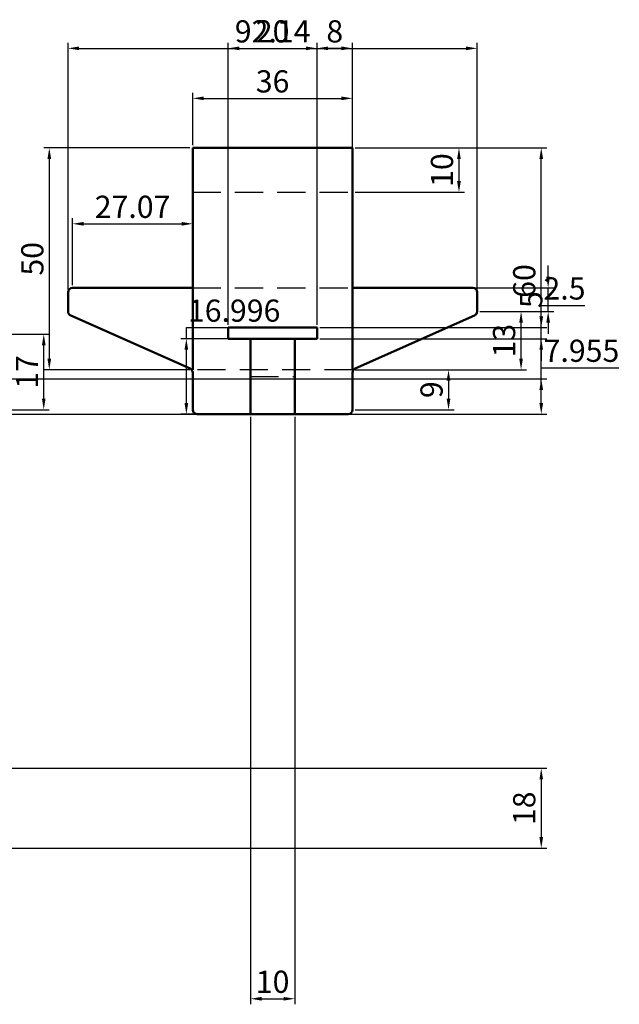
# Model space of a CAD drawing. Units: millimetres. Extents: x 2010 to 2347, y 1200 to 1429.
# Tile 3 of 3: x 2212 to 2347, y 1200 to 1422. Entities that reach past the tile are written whole.
import ezdxf

# ---------------------------------------------------------------- set-up
doc = ezdxf.new("R2010")
doc.units = ezdxf.units.MM
doc.linetypes.add('HIDDEN', pattern=[9.525, 6.35, -3.175])
for name, color, linetype, lineweight in [('M-DIMS', 2, 'Continuous', 25), ('M-HIDN', 3, 'HIDDEN', 25), ('M-OUTL', 7, 'Continuous', 50)]:
    doc.layers.add(name, color=color, linetype=linetype, lineweight=lineweight)
doc.styles.get("Standard").update_dxf_attribs({"font": 'arial.ttf'})
doc.dimstyles.new('ISO-25', dxfattribs={"dimtxt": 5, "dimasz": 2.5, "dimexe": 1.25, "dimexo": 0.625, "dimtad": 1, "dimtoh": 1, "dimdec": 0, "dimtxsty": 'Standard', "dimcen": 2.5, "dimadec": 0, "dimazin": 0, "dimtfac": 1, "dimtdec": 0, "dimtmove": 0, "dimatfit": 3, "dimfxl": 1, "dimarcsym": 0})

# ---------------------------------------------------------------- blocks, each defined once
blk = doc.blocks.new('*D2')
at = {"layer": 'Defpoints', "color": 0, "transparency": 16777216}
for p in [(2196.57, 1351.05), (2217.71, 1351.05), (2197.57, 1334.05)]:
    blk.add_point(p, dxfattribs=at)
at = {"layer": 'M-DIMS', "color": 0, "lineweight": -2, "transparency": 16777216}
for p, q in [((2197.19, 1351.05), (2218.96, 1351.05)), ((2217.71, 1336.55), (2217.71, 1348.55)), ((2198.19, 1334.05), (2218.96, 1334.05))]:
    blk.add_line(p, q, dxfattribs=at)
at = {"layer": 'M-DIMS', "color": 0, "transparency": 16777216}
for points in [[(2217.3, 1348.55), (2218.13, 1348.55), (2217.71, 1351.05)], [(2217.3, 1336.55), (2218.13, 1336.55), (2217.71, 1334.05)]]:
    blk.add_solid(points, dxfattribs=at)
at = {"layer": 'M-DIMS', "color": 0, "transparency": 16777216, "insert": (2214.58, 1342.55), "char_height": 5, "attachment_point": 5, "rotation": 90}
blk.add_mtext('17', dxfattribs=at)
blk = doc.blocks.new('*D17')
at = {"layer": 'Defpoints', "color": 0, "transparency": 16777216}
for p in [(2287.26, 1343.05), (2287.26, 1334.05), (2308.88, 1334.05)]:
    blk.add_point(p, dxfattribs=at)
at = {"layer": 'M-DIMS', "color": 0, "lineweight": -2, "transparency": 16777216}
for p, q in [((2287.89, 1343.05), (2310.13, 1343.05)), ((2308.88, 1340.55), (2308.88, 1336.55)), ((2287.89, 1334.05), (2310.13, 1334.05))]:
    blk.add_line(p, q, dxfattribs=at)
at = {"layer": 'M-DIMS', "color": 0, "transparency": 16777216}
for points in [[(2308.46, 1340.55), (2309.3, 1340.55), (2308.88, 1343.05)], [(2308.46, 1336.55), (2309.3, 1336.55), (2308.88, 1334.05)]]:
    blk.add_solid(points, dxfattribs=at)
at = {"layer": 'M-DIMS', "color": 0, "transparency": 16777216, "insert": (2305.7, 1338.55), "char_height": 5, "attachment_point": 5, "rotation": 90}
blk.add_mtext('9', dxfattribs=at)
blk = doc.blocks.new('*D18')
at = {"layer": 'Defpoints', "color": 0, "transparency": 16777216}
for p in [(2315.33, 1356.16), (2325.22, 1356.16), (2287.26, 1343.05)]:
    blk.add_point(p, dxfattribs=at)
at = {"layer": 'M-DIMS', "color": 0, "lineweight": -2, "transparency": 16777216}
for p, q in [((2315.96, 1356.16), (2326.47, 1356.16)), ((2325.22, 1345.55), (2325.22, 1353.66)), ((2287.89, 1343.05), (2326.47, 1343.05))]:
    blk.add_line(p, q, dxfattribs=at)
at = {"layer": 'M-DIMS', "color": 0, "transparency": 16777216}
for points in [[(2324.8, 1353.66), (2325.63, 1353.66), (2325.22, 1356.16)], [(2324.8, 1345.55), (2325.63, 1345.55), (2325.22, 1343.05)]]:
    blk.add_solid(points, dxfattribs=at)
at = {"layer": 'M-DIMS', "color": 0, "transparency": 16777216, "insert": (2322.04, 1349.6), "char_height": 5, "attachment_point": 5, "rotation": 90}
blk.add_mtext('13', dxfattribs=at)
blk = doc.blocks.new('*D19')
at = {"layer": 'Defpoints', "color": 0, "transparency": 16777216}
for p in [(2314.33, 1361.51), (2331.32, 1361.51), (2315.33, 1356.16)]:
    blk.add_point(p, dxfattribs=at)
at = {"layer": 'M-DIMS', "color": 0, "lineweight": -2, "transparency": 16777216}
for p, q in [((2331.32, 1364.01), (2331.32, 1366.51)), ((2314.96, 1361.51), (2332.57, 1361.51)), ((2331.32, 1356.16), (2331.32, 1361.51)), ((2315.96, 1356.16), (2332.57, 1356.16)), ((2331.32, 1353.66), (2331.32, 1351.16))]:
    blk.add_line(p, q, dxfattribs=at)
at = {"layer": 'M-DIMS', "color": 0, "transparency": 16777216}
for points in [[(2330.9, 1364.01), (2331.73, 1364.01), (2331.32, 1361.51)], [(2330.9, 1353.66), (2331.73, 1353.66), (2331.32, 1356.16)]]:
    blk.add_solid(points, dxfattribs=at)
at = {"layer": 'M-DIMS', "color": 0, "transparency": 16777216, "insert": (2328.15, 1358.84), "char_height": 5, "attachment_point": 5, "rotation": 90}
blk.add_mtext('5', dxfattribs=at)
blk = doc.blocks.new('*D20')
at = {"layer": 'Defpoints', "color": 0, "transparency": 16777216}
for p in [(2287.26, 1393.05), (2287.26, 1383.05), (2311.23, 1383.05)]:
    blk.add_point(p, dxfattribs=at)
at = {"layer": 'M-DIMS', "color": 0, "lineweight": -2, "transparency": 16777216}
for p, q in [((2287.89, 1393.05), (2312.48, 1393.05)), ((2311.23, 1390.55), (2311.23, 1385.55)), ((2287.89, 1383.05), (2312.48, 1383.05))]:
    blk.add_line(p, q, dxfattribs=at)
at = {"layer": 'M-DIMS', "color": 0, "transparency": 16777216}
for points in [[(2310.81, 1390.55), (2311.64, 1390.55), (2311.23, 1393.05)], [(2310.81, 1385.55), (2311.64, 1385.55), (2311.23, 1383.05)]]:
    blk.add_solid(points, dxfattribs=at)
at = {"layer": 'M-DIMS', "color": 0, "transparency": 16777216, "insert": (2308.05, 1388.05), "char_height": 5, "attachment_point": 5, "rotation": 90}
blk.add_mtext('10', dxfattribs=at)
blk = doc.blocks.new('*D21')
at = {"layer": 'Defpoints', "color": 0, "transparency": 16777216}
for p in [(2287.26, 1404.21), (2251.26, 1393.05), (2287.26, 1393.05)]:
    blk.add_point(p, dxfattribs=at)
at = {"layer": 'M-DIMS', "color": 0, "lineweight": -2, "transparency": 16777216}
for p, q in [((2251.26, 1393.67), (2251.26, 1405.46)), ((2287.26, 1393.67), (2287.26, 1405.46)), ((2253.76, 1404.21), (2284.76, 1404.21))]:
    blk.add_line(p, q, dxfattribs=at)
at = {"layer": 'M-DIMS', "color": 0, "transparency": 16777216}
for points in [[(2253.76, 1404.63), (2253.76, 1403.8), (2251.26, 1404.21)], [(2284.76, 1404.63), (2284.76, 1403.8), (2287.26, 1404.21)]]:
    blk.add_solid(points, dxfattribs=at)
at = {"layer": 'M-DIMS', "color": 0, "transparency": 16777216, "insert": (2269.26, 1407.39), "char_height": 5, "attachment_point": 5}
blk.add_mtext('36', dxfattribs=at)
blk = doc.blocks.new('*D22')
at = {"layer": 'Defpoints', "color": 0, "transparency": 16777216}
for p in [(2251.26, 1393.05), (2218.96, 1343.05), (2251.26, 1343.05)]:
    blk.add_point(p, dxfattribs=at)
at = {"layer": 'M-DIMS', "color": 0, "lineweight": -2, "transparency": 16777216}
for p, q in [((2250.64, 1393.05), (2217.71, 1393.05)), ((2218.96, 1390.55), (2218.96, 1345.55)), ((2250.64, 1343.05), (2217.71, 1343.05))]:
    blk.add_line(p, q, dxfattribs=at)
at = {"layer": 'M-DIMS', "color": 0, "transparency": 16777216}
for points in [[(2218.55, 1390.55), (2219.38, 1390.55), (2218.96, 1393.05)], [(2218.55, 1345.55), (2219.38, 1345.55), (2218.96, 1343.05)]]:
    blk.add_solid(points, dxfattribs=at)
at = {"layer": 'M-DIMS', "color": 0, "transparency": 16777216, "insert": (2215.79, 1368.05), "char_height": 5, "attachment_point": 5, "rotation": 90}
blk.add_mtext('50', dxfattribs=at)
blk = doc.blocks.new('*D26')
at = {"layer": 'Defpoints', "color": 0, "transparency": 16777216}
for p in [(2315.33, 1415.48), (2223.19, 1360.51), (2315.33, 1360.51)]:
    blk.add_point(p, dxfattribs=at)
at = {"layer": 'M-DIMS', "color": 0, "lineweight": -2, "transparency": 16777216}
for p, q in [((2223.19, 1361.14), (2223.19, 1416.73)), ((2315.33, 1361.14), (2315.33, 1416.73)), ((2225.69, 1415.48), (2312.83, 1415.48))]:
    blk.add_line(p, q, dxfattribs=at)
at = {"layer": 'M-DIMS', "color": 0, "transparency": 16777216}
for points in [[(2225.69, 1415.9), (2225.69, 1415.06), (2223.19, 1415.48)], [(2312.83, 1415.9), (2312.83, 1415.06), (2315.33, 1415.48)]]:
    blk.add_solid(points, dxfattribs=at)
at = {"layer": 'M-DIMS', "color": 0, "transparency": 16777216, "insert": (2269.26, 1418.66), "char_height": 5, "attachment_point": 5}
blk.add_mtext('92.14', dxfattribs=at)
blk = doc.blocks.new('*D28')
at = {"layer": 'Defpoints', "color": 0, "transparency": 16777216}
for p in [(2279.26, 1415.48), (2259.26, 1352.55), (2279.26, 1352.55)]:
    blk.add_point(p, dxfattribs=at)
at = {"layer": 'M-DIMS', "color": 0, "lineweight": -2, "transparency": 16777216}
for p, q in [((2259.26, 1353.17), (2259.26, 1416.73)), ((2279.26, 1353.17), (2279.26, 1416.73)), ((2261.76, 1415.48), (2276.76, 1415.48))]:
    blk.add_line(p, q, dxfattribs=at)
at = {"layer": 'M-DIMS', "color": 0, "transparency": 16777216}
for points in [[(2261.76, 1415.9), (2261.76, 1415.06), (2259.26, 1415.48)], [(2276.76, 1415.9), (2276.76, 1415.06), (2279.26, 1415.48)]]:
    blk.add_solid(points, dxfattribs=at)
at = {"layer": 'M-DIMS', "color": 0, "transparency": 16777216, "insert": (2269.26, 1418.66), "char_height": 5, "attachment_point": 5}
blk.add_mtext('20', dxfattribs=at)
blk = doc.blocks.new('*D29')
at = {"layer": 'Defpoints', "color": 0, "transparency": 16777216}
for p in [(2264.26, 1333.05), (2274.26, 1333.05), (2274.26, 1201.29)]:
    blk.add_point(p, dxfattribs=at)
at = {"layer": 'M-DIMS', "color": 0, "lineweight": -2, "transparency": 16777216}
for p, q in [((2264.26, 1332.42), (2264.26, 1200.04)), ((2274.26, 1332.42), (2274.26, 1200.04)), ((2266.76, 1201.29), (2271.76, 1201.29))]:
    blk.add_line(p, q, dxfattribs=at)
at = {"layer": 'M-DIMS', "color": 0, "transparency": 16777216}
for points in [[(2266.76, 1201.7), (2266.76, 1200.87), (2264.26, 1201.29)], [(2271.76, 1201.7), (2271.76, 1200.87), (2274.26, 1201.29)]]:
    blk.add_solid(points, dxfattribs=at)
at = {"layer": 'M-DIMS', "color": 0, "transparency": 16777216, "insert": (2269.26, 1204.47), "char_height": 5, "attachment_point": 5}
blk.add_mtext('10', dxfattribs=at)
blk = doc.blocks.new('*D30')
at = {"layer": 'Defpoints', "color": 0, "transparency": 16777216}
for p in [(2279.26, 1352.55), (2329.76, 1352.55), (2279.26, 1350.05)]:
    blk.add_point(p, dxfattribs=at)
at = {"layer": 'M-DIMS', "color": 0, "lineweight": -2, "transparency": 16777216}
for p, q in [((2329.76, 1355.05), (2329.76, 1357.55)), ((2329.76, 1357.55), (2339.61, 1357.55)), ((2279.89, 1352.55), (2331.01, 1352.55)), ((2329.76, 1350.05), (2329.76, 1352.55)), ((2279.89, 1350.05), (2331.01, 1350.05)), ((2329.76, 1347.55), (2329.76, 1345.05))]:
    blk.add_line(p, q, dxfattribs=at)
at = {"layer": 'M-DIMS', "color": 0, "transparency": 16777216}
for points in [[(2329.35, 1355.05), (2330.18, 1355.05), (2329.76, 1352.55)], [(2329.35, 1347.55), (2330.18, 1347.55), (2329.76, 1350.05)]]:
    blk.add_solid(points, dxfattribs=at)
at = {"layer": 'M-DIMS', "color": 0, "transparency": 16777216, "insert": (2335, 1360.72), "char_height": 5, "attachment_point": 5}
blk.add_mtext('2.5', dxfattribs=at)
blk = doc.blocks.new('*D31')
at = {"layer": 'Defpoints', "color": 0, "transparency": 16777216}
for p in [(2249.83, 1350.05), (2264.26, 1350.05), (2264.26, 1333.05)]:
    blk.add_point(p, dxfattribs=at)
at = {"layer": 'M-DIMS', "color": 0, "lineweight": -2, "transparency": 16777216}
for p, q in [((2249.83, 1350.05), (2249.83, 1352.55)), ((2249.83, 1352.55), (2270.74, 1352.55)), ((2263.64, 1350.05), (2248.58, 1350.05)), ((2249.83, 1335.55), (2249.83, 1347.55)), ((2263.64, 1333.05), (2248.58, 1333.05))]:
    blk.add_line(p, q, dxfattribs=at)
at = {"layer": 'M-DIMS', "color": 0, "transparency": 16777216}
for points in [[(2249.41, 1347.55), (2250.25, 1347.55), (2249.83, 1350.05)], [(2249.41, 1335.55), (2250.25, 1335.55), (2249.83, 1333.05)]]:
    blk.add_solid(points, dxfattribs=at)
at = {"layer": 'M-DIMS', "color": 0, "transparency": 16777216, "insert": (2260.6, 1355.72), "char_height": 5, "attachment_point": 5}
blk.add_mtext('16.996', dxfattribs=at)
blk = doc.blocks.new('*D36')
at = {"layer": 'Defpoints', "color": 0, "transparency": 16777216}
for p in [(2106.57, 1341), (2329.76, 1341), (2196.57, 1333.05)]:
    blk.add_point(p, dxfattribs=at)
at = {"layer": 'M-DIMS', "color": 0, "lineweight": -2, "transparency": 16777216}
for p, q in [((2329.76, 1341), (2329.76, 1343.5)), ((2329.76, 1343.5), (2347.26, 1343.5)), ((2107.19, 1341), (2331.01, 1341)), ((2329.76, 1335.55), (2329.76, 1338.5)), ((2197.19, 1333.05), (2331.01, 1333.05))]:
    blk.add_line(p, q, dxfattribs=at)
at = {"layer": 'M-DIMS', "color": 0, "transparency": 16777216}
for points in [[(2329.35, 1338.5), (2330.18, 1338.5), (2329.76, 1341)], [(2329.35, 1335.55), (2330.18, 1335.55), (2329.76, 1333.05)]]:
    blk.add_solid(points, dxfattribs=at)
at = {"layer": 'M-DIMS', "color": 0, "transparency": 16777216, "insert": (2338.82, 1346.68), "char_height": 5, "attachment_point": 5}
blk.add_mtext('7.955', dxfattribs=at)
blk = doc.blocks.new('*D42')
at = {"layer": 'Defpoints', "color": 0, "transparency": 16777216}
for p in [(2287.26, 1393.05), (2329.76, 1393.05), (2286.26, 1333.05)]:
    blk.add_point(p, dxfattribs=at)
at = {"layer": 'M-DIMS', "color": 0, "lineweight": -2, "transparency": 16777216}
for p, q in [((2287.89, 1393.05), (2331.01, 1393.05)), ((2329.76, 1335.55), (2329.76, 1390.55)), ((2286.89, 1333.05), (2331.01, 1333.05))]:
    blk.add_line(p, q, dxfattribs=at)
at = {"layer": 'M-DIMS', "color": 0, "transparency": 16777216}
for points in [[(2329.35, 1390.55), (2330.18, 1390.55), (2329.76, 1393.05)], [(2329.35, 1335.55), (2330.18, 1335.55), (2329.76, 1333.05)]]:
    blk.add_solid(points, dxfattribs=at)
at = {"layer": 'M-DIMS', "color": 0, "transparency": 16777216, "insert": (2326.58, 1363.05), "char_height": 5, "attachment_point": 5, "rotation": 90}
blk.add_mtext('60', dxfattribs=at)
blk = doc.blocks.new('*D43')
at = {"layer": 'Defpoints', "color": 0, "transparency": 16777216}
for p in [(2169.36, 1253.22), (2188.36, 1235.22), (2329.76, 1235.22)]:
    blk.add_point(p, dxfattribs=at)
at = {"layer": 'M-DIMS', "color": 0, "lineweight": -2, "transparency": 16777216}
for p, q in [((2169.98, 1253.22), (2331.01, 1253.22)), ((2329.76, 1250.72), (2329.76, 1237.72)), ((2188.98, 1235.22), (2331.01, 1235.22))]:
    blk.add_line(p, q, dxfattribs=at)
at = {"layer": 'M-DIMS', "color": 0, "transparency": 16777216}
for points in [[(2329.35, 1250.72), (2330.18, 1250.72), (2329.76, 1253.22)], [(2329.35, 1237.72), (2330.18, 1237.72), (2329.76, 1235.22)]]:
    blk.add_solid(points, dxfattribs=at)
at = {"layer": 'M-DIMS', "color": 0, "transparency": 16777216, "insert": (2326.58, 1244.22), "char_height": 5, "attachment_point": 5, "rotation": 90}
blk.add_mtext('18', dxfattribs=at)
blk = doc.blocks.new('*D45')
at = {"layer": 'Defpoints', "color": 0, "transparency": 16777216}
for p in [(2279.26, 1415.48), (2279.26, 1352.55), (2287.26, 1334.05)]:
    blk.add_point(p, dxfattribs=at)
at = {"layer": 'M-DIMS', "color": 0, "lineweight": -2, "transparency": 16777216}
for p, q in [((2279.26, 1353.17), (2279.26, 1416.73)), ((2287.26, 1334.67), (2287.26, 1416.73)), ((2284.76, 1415.48), (2281.76, 1415.48))]:
    blk.add_line(p, q, dxfattribs=at)
at = {"layer": 'M-DIMS', "color": 0, "transparency": 16777216}
for points in [[(2281.76, 1415.9), (2281.76, 1415.06), (2279.26, 1415.48)], [(2284.76, 1415.9), (2284.76, 1415.06), (2287.26, 1415.48)]]:
    blk.add_solid(points, dxfattribs=at)
at = {"layer": 'M-DIMS', "color": 0, "transparency": 16777216, "insert": (2283.26, 1418.66), "char_height": 5, "attachment_point": 5}
blk.add_mtext('8', dxfattribs=at)
blk = doc.blocks.new('*D48')
at = {"layer": 'Defpoints', "color": 0, "transparency": 16777216}
for p in [(2251.26, 1375.94), (2224.19, 1361.51), (2251.26, 1361.51)]:
    blk.add_point(p, dxfattribs=at)
at = {"layer": 'M-DIMS', "color": 0, "lineweight": -2, "transparency": 16777216}
for p, q in [((2224.19, 1362.14), (2224.19, 1377.19)), ((2226.69, 1375.94), (2248.76, 1375.94)), ((2251.26, 1362.14), (2251.26, 1377.19))]:
    blk.add_line(p, q, dxfattribs=at)
at = {"layer": 'M-DIMS', "color": 0, "transparency": 16777216}
for points in [[(2226.69, 1376.36), (2226.69, 1375.52), (2224.19, 1375.94)], [(2248.76, 1376.36), (2248.76, 1375.52), (2251.26, 1375.94)]]:
    blk.add_solid(points, dxfattribs=at)
at = {"layer": 'M-DIMS', "color": 0, "transparency": 16777216, "insert": (2237.72, 1379.12), "char_height": 5, "attachment_point": 5}
blk.add_mtext('27.07', dxfattribs=at)

msp = doc.modelspace()

# ---------------------------------------------------------------- linework, layer by layer
at = {"layer": 'M-HIDN'}
for p, q in [((2251.2603, 1393.0495), (2251.2603, 1383.0495)), ((2251.2603, 1383.0495), (2287.2603, 1383.0495)), ((2251.2603, 1361.5102), (2287.2603, 1361.5102)), ((2287.2603, 1343.0495), (2251.2603, 1343.0495)), ((2264.2603, 1341.5475), (2274.2603, 1341.5475)), ((2274.2603, 1341.5475), (2274.2603, 1341.5475))]:
    msp.add_line(p, q, dxfattribs=at)
at = {"layer": 'M-OUTL'}
for p, q in [((2251.2603, 1343.0495), (2251.2603, 1393.0495)), ((2251.2603, 1393.0495), (2287.2603, 1393.0495)), ((2287.2603, 1393.0495), (2287.2603, 1343.0495)), ((2223.1888, 1356.1604), (2223.1888, 1360.5102)), ((2224.1888, 1361.5102), (2251.2603, 1361.5102)), ((2314.3318, 1361.5102), (2287.2603, 1361.5102)), ((2315.3318, 1356.1604), (2315.3318, 1360.5102)), ((2250.666, 1343.3133), (2223.7831, 1355.2464)), ((2287.8546, 1343.3133), (2314.7375, 1355.2464)), ((2259.2603, 1350.0455), (2259.2603, 1352.5455)), ((2259.2603, 1352.5455), (2279.2603, 1352.5455)), ((2279.2603, 1352.5455), (2279.2603, 1350.0455)), ((2264.2603, 1350.0455), (2259.2603, 1350.0455)), ((2264.2603, 1333.0495), (2264.2603, 1350.0455)), ((2264.2603, 1350.0455), (2274.2603, 1350.0455)), ((2274.2603, 1350.0455), (2274.2603, 1333.0495)), ((2279.2603, 1350.0455), (2274.2603, 1350.0455)), ((2251.2603, 1334.0495), (2251.2603, 1342.3993)), ((2287.2603, 1334.0495), (2287.2603, 1342.3993)), ((2252.2603, 1333.0495), (2286.2603, 1333.0495)), ((2269.2603, 1333.0495), (2264.2603, 1333.0495))]:
    msp.add_line(p, q, dxfattribs=at)
for centre, start, end in [((2224.1888, 1360.5102), 90, 180), ((2314.3318, 1360.5102), 0, 90), ((2224.1888, 1356.1604), 180, 246.063944), ((2314.3318, 1356.1604), 293.936056, 0), ((2250.2603, 1342.3993), 0, 66.063944), ((2288.2603, 1342.3993), 113.936056, 180), ((2252.2603, 1334.0495), 180, 270), ((2286.2603, 1334.0495), 270, 0)]:
    msp.add_arc(centre, 1, start, end, dxfattribs=at)

# ---------------------------------------------------------------- dimensions: what is measured, and where the dimension line sits
at = {"layer": 'M-DIMS'}
for base, p1, p2, override, picture, middle in [((2315.3318, 1415.4795), (2223.1888, 1360.5102), (2315.3318, 1360.5102), {"dimdec": 2, "dimlfac": 1, "dimrnd": 0, "dimzin": 0, "dimdsep": 46, "dimlunit": 2}, '*D26', (2269.2603, 1418.6574)), ((2279.2603, 1415.4795), (2259.2603, 1352.5455), (2279.2603, 1352.5455), {"dimdec": 0, "dimlfac": 1, "dimrnd": 0, "dimzin": 0, "dimdsep": 46, "dimlunit": 2}, '*D28', (2269.2603, 1418.6574)), ((2279.2603, 1415.4795), (2287.2603, 1334.0495), (2279.2603, 1352.5455), {"dimdec": 0, "dimlfac": 1, "dimrnd": 0, "dimzin": 0, "dimdsep": 46, "dimlunit": 2}, '*D45', (2283.2603, 1418.6574)), ((2287.2603, 1404.2128), (2251.2603, 1393.0495), (2287.2603, 1393.0495), {"dimclrd": 0, "dimclre": 0, "dimclrt": 0}, '*D21', (2269.2603, 1407.3924)), ((2274.2603, 1201.2877), (2264.2603, 1333.0495), (2274.2603, 1333.0495), {"dimdec": 0, "dimlfac": 1, "dimrnd": 0, "dimzin": 0, "dimdsep": 46, "dimlunit": 2}, '*D29', (2269.2603, 1204.4655))]:
    dim = msp.add_linear_dim(base=base, p1=p1, p2=p2, dimstyle='ISO-25', override=override, dxfattribs=at)
    dim.commit()
    dim.dimension.update_dxf_attribs({"geometry": picture, "text_midpoint": middle})
for base, p1, p2, angle, override, picture, middle in [((2218.964, 1343.0495), (2251.2603, 1393.0495), (2251.2603, 1343.0495), 90, {"dimclrd": 0, "dimclre": 0, "dimclrt": 0}, '*D22', (2215.7861, 1368.0495)), ((2329.7618, 1393.0495), (2286.2603, 1333.0495), (2287.2603, 1393.0495), 90, {"dimdec": 0, "dimlfac": 1, "dimrnd": 0, "dimzin": 0, "dimdsep": 46, "dimlunit": 2}, '*D42', (2326.5839, 1363.0495)), ((2311.2281, 1383.0495), (2287.2603, 1393.0495), (2287.2603, 1383.0495), 90, {"dimclrd": 0, "dimclre": 0, "dimclrt": 0}, '*D20', (2308.0502, 1388.0495)), ((2251.2603, 1375.9402), (2224.1888, 1361.5102), (2251.2603, 1361.5102), 0, {"dimdec": 2, "dimlfac": 1, "dimrnd": 0, "dimzin": 0, "dimdsep": 46, "dimlunit": 2}, '*D48', (2237.7245, 1379.1181)), ((2331.3162, 1361.5102), (2315.3318, 1356.1604), (2314.3318, 1361.5102), 90, {"dimclrd": 0, "dimclre": 0, "dimclrt": 0}, '*D19', (2328.1486, 1358.8353)), ((2329.7618, 1352.5455), (2279.2603, 1350.0455), (2279.2603, 1352.5455), 90, {"dimdec": 1, "dimlfac": 1, "dimrnd": 0, "dimzin": 0, "dimdsep": 46, "dimlunit": 2}, '*D30', (2334.9997, 1360.7233)), ((2249.8303, 1350.0455), (2264.2603, 1333.0495), (2264.2603, 1350.0455), 90, {"dimdec": 3, "dimlfac": 1, "dimrnd": 0, "dimzin": 0, "dimdsep": 46, "dimlunit": 2}, '*D31', (2260.5968, 1355.7233)), ((2325.2171, 1356.1604), (2287.2603, 1343.0495), (2315.3318, 1356.1604), 90, {"dimclrd": 0, "dimclre": 0, "dimclrt": 0}, '*D18', (2322.0375, 1349.605)), ((2329.7618, 1341.0047), (2196.5687, 1333.0495), (2106.5687, 1341.0047), 90, {"dimdec": 3, "dimlfac": 1, "dimrnd": 0, "dimzin": 0, "dimdsep": 46, "dimlunit": 2}, '*D36', (2338.8213, 1346.6825)), ((2217.714, 1351.0495), (2197.5687, 1334.0495), (2196.5687, 1351.0495), 90, {"dimclrd": 0, "dimclre": 0, "dimclrt": 0}, '*D2', (2214.5787, 1342.5495)), ((2308.8801, 1334.0495), (2287.2603, 1343.0495), (2287.2603, 1334.0495), 90, {"dimclrd": 0, "dimclre": 0, "dimclrt": 0}, '*D17', (2305.7022, 1338.5495)), ((2329.7618, 1235.2177), (2169.3551, 1253.2177), (2188.3551, 1235.2177), 90, {"dimdec": 0, "dimlfac": 1, "dimrnd": 0, "dimzin": 0, "dimdsep": 46, "dimlunit": 2}, '*D43', (2326.5839, 1244.2177))]:
    dim = msp.add_linear_dim(base=base, p1=p1, p2=p2, angle=angle, dimstyle='ISO-25', override=override, dxfattribs=at)
    dim.commit()
    dim.dimension.update_dxf_attribs({"geometry": picture, "text_midpoint": middle})

doc.saveas('drawing.dxf')
